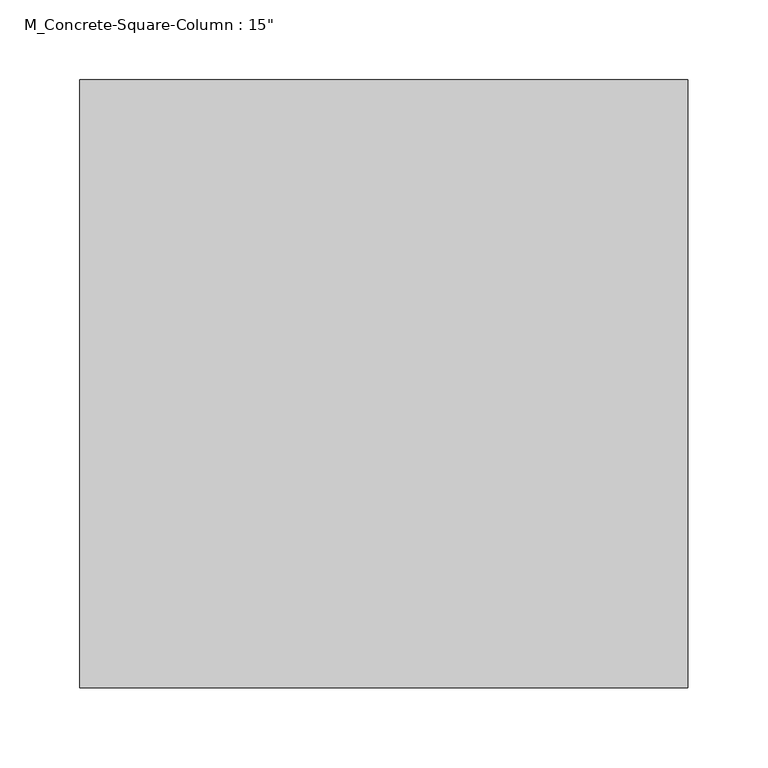
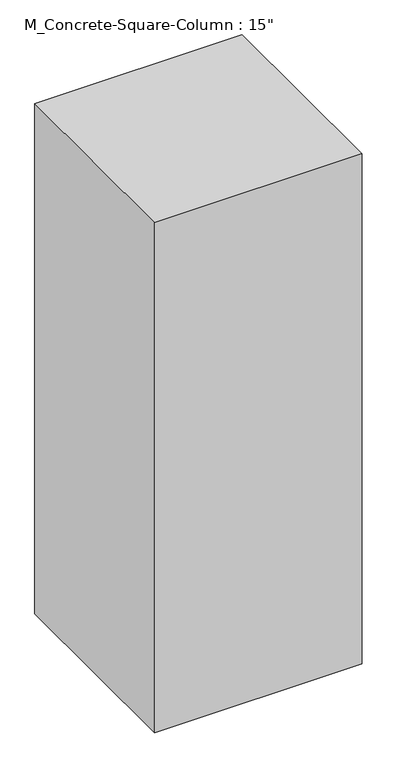
"""IFC4 building model written with IfcOpenShell, lengths in millimetres: column geometry."""

from ifc_helpers import new_model, si_unit, frame, origin, place, context, project, spatial, polyline, outline, extrude, source, transform, mapped, element, save


def column_96418790(model_context):
    return source(origin(), model_context, "Body", "SweptSolid", [
        extrude(outline(polyline([(190.5, 190.5), (190.5, -190.5), (-190.5, -190.5), (-190.5, 190.5), (190.5, 190.5)])), frame((0.0, 0.0, -2133.6), z_axis=(0.0, 0.0, 1.0), x_axis=(1.0, 0.0, 0.0)), (0.0, 0.0, 1.0), 990.6),
    ])


if __name__ == "__main__":
    model = new_model("IFC4")
    model_context = context("Model", 3, world=origin())
    ifc_project = project(units=[si_unit("LENGTHUNIT", "METRE", prefix="MILLI")], contexts=[model_context])
    site = spatial("IfcSite", under=ifc_project)
    building = spatial("IfcBuilding", under=site)
    placement = place(None, origin())
    column_shape = column_96418790(model_context)
    element("IfcColumn", 1, ObjectType="M_Concrete-Square-Column : 15\"", at=placement, inside=building, context=model_context, shape_type="MappedRepresentation", body=[
        mapped(column_shape, transform((0.0, 0.0, 0.0), x_axis=(1.0, 0.0, 0.0), y_axis=(0.0, 1.0, 0.0), z_axis=(0.0, 0.0, 1.0))),
    ])
    save(model, "model.ifc")

# Revit data of these elements
# Type "M_Concrete-Square-Column : 15\""
#   b = 381 mm
#   Structural Material [instance default] = Concrete, Cast-in-Place gray
# Element 1 (IfcColumn, "M_Concrete-Square-Column : 15\"")
#   Materials on its faces: "Concrete, Cast-in-Place gray"
# Materials
#   "Concrete, Cast-in-Place gray": class "Concrete", colour RGB 192 192 192, transparency 0, Description = "Cast-in-place concrete", Cost = 0
